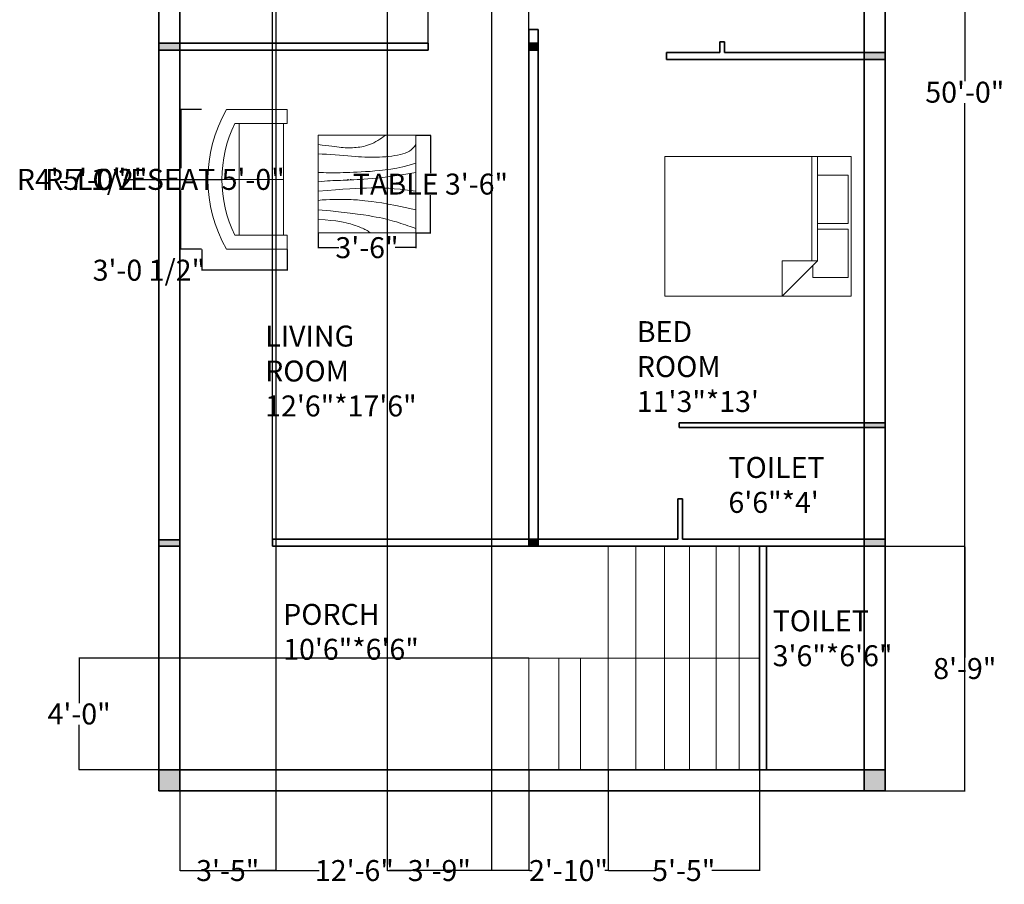
# Model space of a CAD drawing. Units: inches. Extents: x 23641 to 24129, y 27170 to 27889.
# Tile 1 of 2: x 23641 to 24064, y 27170 to 27541. Entities that reach past the tile are written whole.
import ezdxf

# ---------------------------------------------------------------- set-up
doc = ezdxf.new("R2010")
doc.units = ezdxf.units.IN
doc.header["$MEASUREMENT"] = 0
for name, color, linetype, lineweight in [('A-ANNO-DIMS', 2, 'Continuous', 18), ('A-AREA-IDEN', 7, 'Continuous', 25), ('A-FLOR-STRS', 7, 'Continuous', 18), ('A-FURN', 8, 'Continuous', 18), ('A-WALL', 7, 'Continuous', 35), ('A-WALL-PATT', 7, 'Continuous', 13)]:
    doc.layers.add(name, color=color, linetype=linetype, lineweight=lineweight)
doc.styles.get("Standard").update_dxf_attribs({"font": 'arial.ttf'})
doc.dimstyles.get("Standard").update_dxf_attribs({"dimtxt": 9, "dimasz": 0.18, "dimexe": 0.18, "dimexo": 0.0625, "dimgap": 0.09, "dimtad": 0, "dimtih": 1, "dimtoh": 1, "dimdec": 0, "dimzin": 0, "dimdsep": 46, "dimlunit": 3, "dimtxsty": 'Standard', "dimcen": 0.09, "dimadec": 0, "dimazin": 0, "dimtfac": 1, "dimtdec": 0, "dimtofl": 0, "dimtmove": 0, "dimatfit": 3, "dimfxl": 1, "dimtolj": 1, "dimtzin": 0, "dimarcsym": 0})

# ---------------------------------------------------------------- blocks, each defined once
blk = doc.blocks.new('Table - Square Woodgrain 42 x 42 in.')
blk.add_line((0, -42), (42, -42))
for points in [[(0, -4), (1.704, -4.2172), (3.2358, -4.4188), (4.615, -4.604), (5.8615, -4.7721), (6.9951, -4.9224), (8.0357, -5.0541), (9.0031, -5.1667), (9.9171, -5.2594), (10.7951, -5.3316), (11.6445, -5.3836), (12.4702, -5.4157), (13.277, -5.4283), (14.0698, -5.4217), (14.8535, -5.3964), (15.6331, -5.3526), (16.4133, -5.2908), (17.1986, -5.2103), (17.9913, -5.1062), (18.793, -4.9727), (19.6056, -4.8038), (20.4307, -4.5937), (21.2701, -4.3365), (22.1256, -4.0262), (22.9989, -3.6571), (23.888, -3.2272), (24.7756, -2.7516), (25.6408, -2.2491), (26.4624, -1.7387), (27.2195, -1.2395), (27.891, -0.7703), (28.456, -0.3501), (28.8934, 0.002)], [(0, -42), (0, 0), (42, 0), (42, -42)], [(0, -8), (1.8203, -8.1001), (3.6741, -8.2149), (5.5411, -8.3408), (7.4011, -8.4741), (9.2339, -8.6112), (11.0193, -8.7484), (12.7371, -8.8821), (14.3671, -9.0086), (15.8954, -9.1246), (17.3337, -9.2278), (18.6997, -9.3159), (20.0116, -9.387), (21.2871, -9.4389), (22.5442, -9.4696), (23.8008, -9.477), (25.0749, -9.459), (26.3791, -9.4137), (27.7049, -9.3403), (29.0383, -9.2382), (30.3655, -9.1068), (31.6728, -8.9455), (32.9461, -8.7535), (34.1717, -8.5304), (35.3358, -8.2756), (36.4268, -7.9863), (37.443, -7.6521), (38.3849, -7.2603), (39.253, -6.7986), (40.048, -6.2542), (40.7705, -5.6147), (41.421, -4.8674), (42, -4)], [(42, -12), (39.1784, -12.8621), (36.4519, -13.5654), (33.8246, -14.1294), (31.3004, -14.5731), (28.8832, -14.9161), (26.577, -15.1775), (24.3858, -15.3768), (22.3136, -15.5332), (20.3622, -15.6632), (18.5254, -15.7718), (16.7947, -15.8612), (15.1618, -15.9338), (13.6183, -15.9916), (12.1558, -16.0369), (10.7659, -16.0718), (9.4403, -16.0987), (8.1703, -16.1191), (6.9461, -16.1325), (5.7577, -16.1377), (4.595, -16.1335), (3.4479, -16.1188), (2.3064, -16.0924), (1.1604, -16.0532), (0, -16)], [(42, -16), (37.6529, -16.7365), (33.8802, -17.329), (30.6179, -17.7961), (27.8015, -18.1561), (25.3668, -18.4275), (23.2497, -18.6288), (21.3859, -18.7785), (19.7111, -18.8949), (18.1693, -18.9939), (16.7375, -19.0795), (15.401, -19.1534), (14.1449, -19.217), (12.9544, -19.2717), (11.8148, -19.3191), (10.7113, -19.3606), (9.6291, -19.3976), (8.5534, -19.4323), (7.47, -19.4689), (6.3643, -19.5122), (5.222, -19.5672), (4.0288, -19.6386), (2.7703, -19.7313), (1.4321, -19.8501), (0, -20)], [(0, -24), (3.9243, -23.6805), (7.4766, -23.4138), (10.6891, -23.1954), (13.5943, -23.0205), (16.2247, -22.8847), (18.6125, -22.7832), (20.7903, -22.7116), (22.7903, -22.6651), (24.6563, -22.642), (26.4764, -22.6507), (28.35, -22.7024), (30.3766, -22.8084), (32.6555, -22.98), (35.2861, -23.2283), (38.3678, -23.5645), (42, -24)], [(42, -32), (37.392, -31.017), (33.4585, -30.2231), (30.1291, -29.5949), (27.3334, -29.109), (25.0009, -28.742), (23.0612, -28.4707), (21.4439, -28.2716), (20.0786, -28.1215), (18.8998, -28.0002), (17.8609, -27.9014), (16.9206, -27.8219), (16.0371, -27.7588), (15.1691, -27.709), (14.2748, -27.6693), (13.3128, -27.6368), (12.2415, -27.6083), (11.0295, -27.5824), (9.6867, -27.5643), (8.233, -27.5608), (6.6884, -27.5787), (5.0728, -27.6248), (3.4062, -27.7058), (1.7086, -27.8286), (0, -28)], [(0, -32), (5.4026, -32.5358), (9.9494, -33.019), (13.7424, -33.4553), (16.8834, -33.8505), (19.4743, -34.2106), (21.6171, -34.5413), (23.4136, -34.8486), (24.9657, -35.1382), (26.3614, -35.4156), (27.6332, -35.6841), (28.7995, -35.9467), (29.8788, -36.2064), (30.8897, -36.4661), (31.8507, -36.7288), (32.7802, -36.9973), (33.6968, -37.2747), (34.6175, -37.5635), (35.5531, -37.8651), (36.5128, -38.1805), (37.506, -38.5108), (38.5421, -38.8568), (39.6302, -39.2197), (40.7797, -39.6004), (42, -40)], [(0, -36), (3.0098, -36.2857), (5.5354, -36.5643), (7.6368, -36.8359), (9.374, -37.1009), (10.807, -37.3597), (11.9957, -37.6126), (13.0002, -37.8599), (13.8804, -38.102), (14.6874, -38.3393), (15.4365, -38.5729), (16.1338, -38.8041), (16.7858, -39.0341), (17.3987, -39.264), (17.9787, -39.4952), (18.5322, -39.7288), (19.0655, -39.9662), (19.5832, -40.2081), (20.0842, -40.4544), (20.5657, -40.7046), (21.0249, -40.9581), (21.459, -41.2144), (21.8653, -41.4731), (22.2409, -41.7335), (22.5831, -41.9951)]]:
    blk.add_lwpolyline(points)
blk = doc.blocks.new('Sofa - Roundback Loveseat 5 ft.')
for p, q in [((0, -32.44198), (0, -5.99998)), ((-24, -33.99998), (-24, -11.46958)), ((24.00004, -33.99998), (24.00004, -11.46958)), ((-23.9998, -13.38178), (23.99986, -13.38178)), ((-24, -32.44198), (24.00004, -32.44198))]:
    blk.add_line(p, q)
for points in [[(-24, -33.99998), (-30, -33.99998), (-30, -7.99998)], [(30.00004, -7.99998), (30.00004, -33.99998), (24.00004, -33.99998)]]:
    blk.add_lwpolyline(points)
for centre, radius, start, end in [((0, -60.24998), 60.24998, 60.13715, 119.8628), ((0, -61.38438), 55.38444, 64.32083, 115.6792)]:
    blk.add_arc(centre, radius, start, end)
blk = doc.blocks.new('Bed - Queen')
for p, q in [((0, -80.00003), (0, 0)), ((0, 0), (59.99999, 0)), ((59.99999, 0), (59.99999, -80.00003)), ((7.99999, -1.2), (28.79998, -1.2)), ((7.99999, -14.4), (7.99999, -1.2)), ((28.79998, -1.2), (28.79998, -14.4)), ((31.19999, -1.2), (51.99999, -1.2)), ((31.19999, -14.4), (31.19999, -1.2)), ((51.99999, -1.2), (51.99999, -16.4)), ((0, -14.4), (44.8, -14.4)), ((44.8, -16.8), (0, -16.8)), ((59.99999, -29.6), (44.8, -14.4)), ((44.8, -14.4), (44.8, -29.6)), ((51.99999, -16.4), (46.79936, -16.4)), ((44.8, -29.6), (59.99999, -29.6)), ((59.99999, -80.00003), (0, -80.00003))]:
    blk.add_line(p, q)
blk = doc.blocks.new('*D17')
at = {"layer": 'A-ANNO-DIMS', "color": 0, "lineweight": -2, "transparency": 16777216}
for p, q in [((23811.46, 27491.81), (23817.87, 27491.81)), ((23817.69, 27491.63), (23817.69, 27475.5)), ((23817.69, 27449.99), (23817.69, 27466.12)), ((23811.46, 27449.81), (23817.87, 27449.81))]:
    blk.add_line(p, q, dxfattribs=at)
at = {"layer": 'A-ANNO-DIMS', "color": 0, "transparency": 16777216}
for points in [[(23817.66, 27491.63), (23817.72, 27491.63), (23817.69, 27491.81)], [(23817.66, 27449.99), (23817.72, 27449.99), (23817.69, 27449.81)]]:
    blk.add_solid(points, dxfattribs=at)
at = {"layer": 'Defpoints', "color": 0, "transparency": 16777216}
for p in [(23811.39, 27491.81), (23817.69, 27491.81), (23811.39, 27449.81)]:
    blk.add_point(p, dxfattribs=at)
at = {"layer": 'A-ANNO-DIMS', "color": 0, "transparency": 16777216, "insert": (23817.69, 27470.81), "char_height": 9, "attachment_point": 5}
blk.add_mtext('\\A1;TABLE 3\'-6"', dxfattribs=at)
blk = doc.blocks.new('*D18')
at = {"layer": 'A-ANNO-DIMS', "color": 0, "lineweight": -2, "transparency": 16777216}
for p, q in [((23769.39, 27449.74), (23769.39, 27443.33)), ((23811.39, 27449.74), (23811.39, 27443.33)), ((23769.57, 27443.51), (23778.34, 27443.51)), ((23811.21, 27443.51), (23802.44, 27443.51))]:
    blk.add_line(p, q, dxfattribs=at)
at = {"layer": 'A-ANNO-DIMS', "color": 0, "transparency": 16777216}
for points in [[(23769.57, 27443.54), (23769.57, 27443.48), (23769.39, 27443.51)], [(23811.21, 27443.54), (23811.21, 27443.48), (23811.39, 27443.51)]]:
    blk.add_solid(points, dxfattribs=at)
at = {"layer": 'Defpoints', "color": 0, "transparency": 16777216}
for p in [(23769.39, 27449.81), (23811.39, 27449.81), (23811.39, 27443.51)]:
    blk.add_point(p, dxfattribs=at)
at = {"layer": 'A-ANNO-DIMS', "color": 0, "transparency": 16777216, "insert": (23790.39, 27443.51), "char_height": 9, "attachment_point": 5}
blk.add_mtext('\\A1;3\'-6"', dxfattribs=at)
blk = doc.blocks.new('*D19')
at = {"layer": 'A-ANNO-DIMS', "color": 0, "lineweight": -2, "transparency": 16777216}
for p, q in [((23719.36, 27502.83), (23710.24, 27502.83)), ((23710.42, 27502.65), (23710.42, 27477.58)), ((23710.42, 27443.01), (23710.42, 27468.08)), ((23719.36, 27442.83), (23710.24, 27442.83))]:
    blk.add_line(p, q, dxfattribs=at)
at = {"layer": 'A-ANNO-DIMS', "color": 0, "transparency": 16777216}
for points in [[(23710.39, 27502.65), (23710.45, 27502.65), (23710.42, 27502.83)], [(23710.39, 27443.01), (23710.45, 27443.01), (23710.42, 27442.83)]]:
    blk.add_solid(points, dxfattribs=at)
at = {"layer": 'Defpoints', "color": 0, "transparency": 16777216}
for p in [(23710.42, 27502.83), (23719.42, 27502.83), (23719.42, 27442.83)]:
    blk.add_point(p, dxfattribs=at)
at = {"layer": 'A-ANNO-DIMS', "color": 0, "transparency": 16777216, "insert": (23710.42, 27472.83), "char_height": 9, "attachment_point": 5}
blk.add_mtext('\\A1;LOVESEAT 5\'-0"', dxfattribs=at)
blk = doc.blocks.new('*D20')
at = {"layer": 'A-ANNO-DIMS', "color": 0, "lineweight": -2, "transparency": 16777216}
for p, q in [((23719.42, 27442.77), (23719.42, 27433.65)), ((23756.08, 27442.77), (23756.08, 27433.65)), ((23719.42, 27433.83), (23719.24, 27433.83)), ((23755.9, 27433.83), (23719.6, 27433.83))]:
    blk.add_line(p, q, dxfattribs=at)
at = {"layer": 'A-ANNO-DIMS', "color": 0, "transparency": 16777216}
for points in [[(23719.6, 27433.86), (23719.6, 27433.8), (23719.42, 27433.83)], [(23755.9, 27433.86), (23755.9, 27433.8), (23756.08, 27433.83)]]:
    blk.add_solid(points, dxfattribs=at)
at = {"layer": 'Defpoints', "color": 0, "transparency": 16777216}
for p in [(23719.42, 27442.83), (23756.08, 27442.83), (23719.42, 27433.83)]:
    blk.add_point(p, dxfattribs=at)
at = {"layer": 'A-ANNO-DIMS', "color": 0, "transparency": 16777216, "insert": (23696.7, 27433.83), "char_height": 9, "attachment_point": 5}
blk.add_mtext('\\A1;3\'-0 1/2"', dxfattribs=at)
blk = doc.blocks.new('*D23')
at = {"layer": 'A-ANNO-DIMS', "color": 0, "lineweight": -2, "transparency": 16777216}
for p, q in [((24013.05, 27810.27), (24047.41, 27810.27)), ((24047.23, 27810.09), (24047.23, 27514.96)), ((24047.23, 27210.45), (24047.23, 27505.59)), ((24013.05, 27210.27), (24047.41, 27210.27))]:
    blk.add_line(p, q, dxfattribs=at)
at = {"layer": 'A-ANNO-DIMS', "color": 0, "transparency": 16777216}
for points in [[(24047.2, 27810.09), (24047.26, 27810.09), (24047.23, 27810.27)], [(24047.2, 27210.45), (24047.26, 27210.45), (24047.23, 27210.27)]]:
    blk.add_solid(points, dxfattribs=at)
at = {"layer": 'Defpoints', "color": 0, "transparency": 16777216}
for p in [(24012.98, 27810.27), (24047.23, 27810.27), (24012.98, 27210.27)]:
    blk.add_point(p, dxfattribs=at)
at = {"layer": 'A-ANNO-DIMS', "color": 0, "transparency": 16777216, "insert": (24047.23, 27510.27), "char_height": 9, "attachment_point": 5}
blk.add_mtext('\\A1;50\'-0"', dxfattribs=at)
blk = doc.blocks.new('*D25')
at = {"layer": 'A-ANNO-DIMS', "color": 0, "lineweight": -2, "transparency": 16777216}
for p, q in [((23709.98, 27315.33), (23709.98, 27844.7)), ((23710.16, 27844.52), (23717.83, 27844.52)), ((23749.6, 27844.52), (23741.93, 27844.52)), ((23749.78, 27315.33), (23749.78, 27844.7))]:
    blk.add_line(p, q, dxfattribs=at)
at = {"layer": 'A-ANNO-DIMS', "color": 0, "transparency": 16777216}
for points in [[(23710.16, 27844.55), (23710.16, 27844.49), (23709.98, 27844.52)], [(23749.6, 27844.55), (23749.6, 27844.49), (23749.78, 27844.52)]]:
    blk.add_solid(points, dxfattribs=at)
at = {"layer": 'Defpoints', "color": 0, "transparency": 16777216}
for p in [(23749.78, 27844.52), (23709.98, 27315.27), (23749.78, 27315.27)]:
    blk.add_point(p, dxfattribs=at)
at = {"layer": 'A-ANNO-DIMS', "color": 0, "transparency": 16777216, "insert": (23729.88, 27844.52), "char_height": 9, "attachment_point": 5}
blk.add_mtext('\\A1;3\'-4"', dxfattribs=at)
blk = doc.blocks.new('*D26')
at = {"layer": 'A-ANNO-DIMS', "color": 0, "lineweight": -2, "transparency": 16777216}
for p, q in [((24013.05, 27315.27), (24047.41, 27315.27)), ((24047.23, 27315.09), (24047.23, 27267.46)), ((24047.23, 27210.45), (24047.23, 27258.09)), ((24013.05, 27210.27), (24047.41, 27210.27))]:
    blk.add_line(p, q, dxfattribs=at)
at = {"layer": 'A-ANNO-DIMS', "color": 0, "transparency": 16777216}
for points in [[(24047.2, 27315.09), (24047.26, 27315.09), (24047.23, 27315.27)], [(24047.2, 27210.45), (24047.26, 27210.45), (24047.23, 27210.27)]]:
    blk.add_solid(points, dxfattribs=at)
at = {"layer": 'Defpoints', "color": 0, "transparency": 16777216}
for p in [(24012.98, 27315.27), (24047.23, 27315.27), (24012.98, 27210.27)]:
    blk.add_point(p, dxfattribs=at)
at = {"layer": 'A-ANNO-DIMS', "color": 0, "transparency": 16777216, "insert": (24047.23, 27262.77), "char_height": 9, "attachment_point": 5}
blk.add_mtext('\\A1;8\'-9"', dxfattribs=at)
blk = doc.blocks.new('*D27')
at = {"layer": 'A-ANNO-DIMS', "color": 0, "lineweight": -2, "transparency": 16777216}
for p, q in [((23893.98, 27219.21), (23893.98, 27175.84)), ((23958.98, 27219.21), (23958.98, 27175.84)), ((23894.16, 27176.02), (23914.43, 27176.02)), ((23958.8, 27176.02), (23938.54, 27176.02))]:
    blk.add_line(p, q, dxfattribs=at)
at = {"layer": 'A-ANNO-DIMS', "color": 0, "transparency": 16777216}
for points in [[(23894.16, 27176.05), (23894.16, 27175.99), (23893.98, 27176.02)], [(23958.8, 27176.05), (23958.8, 27175.99), (23958.98, 27176.02)]]:
    blk.add_solid(points, dxfattribs=at)
at = {"layer": 'Defpoints', "color": 0, "transparency": 16777216}
for p in [(23893.98, 27219.27), (23958.98, 27219.27), (23958.98, 27176.02)]:
    blk.add_point(p, dxfattribs=at)
at = {"layer": 'A-ANNO-DIMS', "color": 0, "transparency": 16777216, "insert": (23926.48, 27176.02), "char_height": 9, "attachment_point": 5}
blk.add_mtext('\\A1;5\'-5"', dxfattribs=at)
blk = doc.blocks.new('*D29')
at = {"layer": 'A-ANNO-DIMS', "color": 0, "lineweight": -2, "transparency": 16777216}
for p, q in [((23799.02, 27654.21), (23799.02, 27175.84)), ((23843.92, 27654.21), (23843.92, 27175.84)), ((23799.2, 27176.02), (23809.42, 27176.02)), ((23843.74, 27176.02), (23833.52, 27176.02))]:
    blk.add_line(p, q, dxfattribs=at)
at = {"layer": 'A-ANNO-DIMS', "color": 0, "transparency": 16777216}
for points in [[(23799.2, 27176.05), (23799.2, 27175.99), (23799.02, 27176.02)], [(23843.74, 27176.05), (23843.74, 27175.99), (23843.92, 27176.02)]]:
    blk.add_solid(points, dxfattribs=at)
at = {"layer": 'Defpoints', "color": 0, "transparency": 16777216}
for p in [(23799.02, 27654.27), (23843.92, 27654.27), (23843.92, 27176.02)]:
    blk.add_point(p, dxfattribs=at)
at = {"layer": 'A-ANNO-DIMS', "color": 0, "transparency": 16777216, "insert": (23821.47, 27176.02), "char_height": 9, "attachment_point": 5}
blk.add_mtext('\\A1;3\'-9"', dxfattribs=at)
blk = doc.blocks.new('*D30')
at = {"layer": 'A-ANNO-DIMS', "color": 0, "lineweight": -2, "transparency": 16777216}
for p, q in [((23709.98, 27657.21), (23709.98, 27175.84)), ((23751.17, 27657.21), (23751.17, 27175.84)), ((23710.16, 27176.02), (23718.53, 27176.02)), ((23750.99, 27176.02), (23742.63, 27176.02))]:
    blk.add_line(p, q, dxfattribs=at)
at = {"layer": 'A-ANNO-DIMS', "color": 0, "transparency": 16777216}
for points in [[(23710.16, 27176.05), (23710.16, 27175.99), (23709.98, 27176.02)], [(23750.99, 27176.05), (23750.99, 27175.99), (23751.17, 27176.02)]]:
    blk.add_solid(points, dxfattribs=at)
at = {"layer": 'Defpoints', "color": 0, "transparency": 16777216}
for p in [(23709.98, 27657.27), (23751.17, 27657.27), (23751.17, 27176.02)]:
    blk.add_point(p, dxfattribs=at)
at = {"layer": 'A-ANNO-DIMS', "color": 0, "transparency": 16777216, "insert": (23730.58, 27176.02), "char_height": 9, "attachment_point": 5}
blk.add_mtext('\\A1;3\'-5"', dxfattribs=at)
blk = doc.blocks.new('*D32')
at = {"layer": 'A-ANNO-DIMS', "color": 0, "lineweight": -2, "transparency": 16777216}
for p, q in [((23859.92, 27267.27), (23666.55, 27267.27)), ((23666.73, 27267.09), (23666.73, 27247.96)), ((23666.73, 27219.45), (23666.73, 27238.59)), ((23859.92, 27219.27), (23666.55, 27219.27))]:
    blk.add_line(p, q, dxfattribs=at)
at = {"layer": 'A-ANNO-DIMS', "color": 0, "transparency": 16777216}
for points in [[(23666.7, 27267.09), (23666.76, 27267.09), (23666.73, 27267.27)], [(23666.7, 27219.45), (23666.76, 27219.45), (23666.73, 27219.27)]]:
    blk.add_solid(points, dxfattribs=at)
at = {"layer": 'Defpoints', "color": 0, "transparency": 16777216}
for p in [(23666.73, 27267.27), (23859.98, 27267.27), (23859.98, 27219.27)]:
    blk.add_point(p, dxfattribs=at)
at = {"layer": 'A-ANNO-DIMS', "color": 0, "transparency": 16777216, "insert": (23666.73, 27243.27), "char_height": 9, "attachment_point": 5}
blk.add_mtext('\\A1;4\'-0"', dxfattribs=at)
blk = doc.blocks.new('*D33')
at = {"layer": 'A-ANNO-DIMS', "color": 0, "lineweight": -2, "transparency": 16777216}
for p, q in [((23859.98, 27219.21), (23859.98, 27175.84)), ((23893.98, 27219.21), (23893.98, 27175.84)), ((23860.16, 27176.02), (23861.36, 27176.02)), ((23893.8, 27176.02), (23892.61, 27176.02))]:
    blk.add_line(p, q, dxfattribs=at)
at = {"layer": 'A-ANNO-DIMS', "color": 0, "transparency": 16777216}
for points in [[(23860.16, 27176.05), (23860.16, 27175.99), (23859.98, 27176.02)], [(23893.8, 27176.05), (23893.8, 27175.99), (23893.98, 27176.02)]]:
    blk.add_solid(points, dxfattribs=at)
at = {"layer": 'Defpoints', "color": 0, "transparency": 16777216}
for p in [(23859.98, 27219.27), (23893.98, 27219.27), (23893.98, 27176.02)]:
    blk.add_point(p, dxfattribs=at)
at = {"layer": 'A-ANNO-DIMS', "color": 0, "transparency": 16777216, "insert": (23876.98, 27176.02), "char_height": 9, "attachment_point": 5}
blk.add_mtext('\\A1;2\'-10"', dxfattribs=at)
blk = doc.blocks.new('*D34')
at = {"layer": 'A-ANNO-DIMS', "color": 0, "lineweight": -2, "transparency": 16777216}
for p, q in [((23709.98, 27219.21), (23709.98, 27175.84)), ((23859.98, 27219.21), (23859.98, 27175.84)), ((23710.16, 27176.02), (23769.86, 27176.02)), ((23859.8, 27176.02), (23800.11, 27176.02))]:
    blk.add_line(p, q, dxfattribs=at)
at = {"layer": 'A-ANNO-DIMS', "color": 0, "transparency": 16777216}
for points in [[(23710.16, 27176.05), (23710.16, 27175.99), (23709.98, 27176.02)], [(23859.8, 27176.05), (23859.8, 27175.99), (23859.98, 27176.02)]]:
    blk.add_solid(points, dxfattribs=at)
at = {"layer": 'Defpoints', "color": 0, "transparency": 16777216}
for p in [(23709.98, 27219.27), (23859.98, 27219.27), (23859.98, 27176.02)]:
    blk.add_point(p, dxfattribs=at)
at = {"layer": 'A-ANNO-DIMS', "color": 0, "transparency": 16777216, "insert": (23784.98, 27176.02), "char_height": 9, "attachment_point": 5}
blk.add_mtext('\\A1;12\'-6"', dxfattribs=at)
blk = doc.blocks.new('*D35')
at = {"layer": 'A-ANNO-DIMS', "color": 0, "lineweight": -2, "transparency": 16777216}
for p, q in [((23816.62, 27531.33), (23816.62, 27844.7)), ((23816.8, 27844.52), (23859.8, 27844.52)), ((23859.98, 27531.33), (23859.98, 27844.7)), ((23859.98, 27844.52), (23860.16, 27844.52))]:
    blk.add_line(p, q, dxfattribs=at)
at = {"layer": 'A-ANNO-DIMS', "color": 0, "transparency": 16777216}
for points in [[(23816.8, 27844.55), (23816.8, 27844.49), (23816.62, 27844.52)], [(23859.8, 27844.55), (23859.8, 27844.49), (23859.98, 27844.52)]]:
    blk.add_solid(points, dxfattribs=at)
at = {"layer": 'Defpoints', "color": 0, "transparency": 16777216}
for p in [(23859.98, 27844.52), (23816.62, 27531.27), (23859.98, 27531.27)]:
    blk.add_point(p, dxfattribs=at)
at = {"layer": 'A-ANNO-DIMS', "color": 0, "transparency": 16777216, "insert": (23882.7, 27844.52), "char_height": 9, "attachment_point": 5}
blk.add_mtext('\\A1;3\'-7 1/2"', dxfattribs=at)
blk = doc.blocks.new('*D36')
at = {"layer": 'A-ANNO-DIMS', "color": 0, "lineweight": -2, "transparency": 16777216}
for p, q in [((23685.94, 27472.83), (23721.91, 27472.83)), ((23782.24, 27472.83), (23782.42, 27472.83)), ((23782.33, 27472.74), (23782.33, 27472.92))]:
    blk.add_line(p, q, dxfattribs=at)
at = {"layer": 'A-ANNO-DIMS', "color": 0, "transparency": 16777216}
blk.add_solid([(23721.91, 27472.86), (23721.91, 27472.8), (23722.09, 27472.83)], dxfattribs=at)
at = {"layer": 'Defpoints', "color": 0, "transparency": 16777216}
for p in [(23722.09, 27472.83), (23782.33, 27472.83)]:
    blk.add_point(p, dxfattribs=at)
at = {"layer": 'A-ANNO-DIMS', "color": 0, "transparency": 16777216, "insert": (23669.58, 27472.83), "char_height": 9, "attachment_point": 5}
blk.add_mtext('\\A1;R5\'-0"', dxfattribs=at)
blk = doc.blocks.new('*D37')
at = {"layer": 'A-ANNO-DIMS', "color": 0, "lineweight": -2, "transparency": 16777216}
for p, q in [((23694.85, 27472.83), (23727.9, 27472.83)), ((23783.38, 27472.83), (23783.56, 27472.83)), ((23783.47, 27472.74), (23783.47, 27472.92))]:
    blk.add_line(p, q, dxfattribs=at)
at = {"layer": 'A-ANNO-DIMS', "color": 0, "transparency": 16777216}
blk.add_solid([(23727.9, 27472.86), (23727.9, 27472.8), (23728.08, 27472.83)], dxfattribs=at)
at = {"layer": 'Defpoints', "color": 0, "transparency": 16777216}
for p in [(23728.08, 27472.83), (23783.47, 27472.83)]:
    blk.add_point(p, dxfattribs=at)
at = {"layer": 'A-ANNO-DIMS', "color": 0, "transparency": 16777216, "insert": (23668.01, 27472.83), "char_height": 9, "attachment_point": 5}
blk.add_mtext('\\A1;R4\'-7 1/2"', dxfattribs=at)

msp = doc.modelspace()

# ---------------------------------------------------------------- hatches: boundary and pattern name
at = {"layer": 'A-WALL-PATT'}
h = msp.add_hatch(color=256, dxfattribs=at)
h.dxf.hatch_style = 1
h.paths.add_polyline_path([(23709.98, 27531.27), (23700.98, 27531.27), (23700.98, 27528.27), (23709.98, 27528.27)])
h = msp.add_hatch(color=256, dxfattribs=at)
h.dxf.hatch_style = 1
h.paths.add_polyline_path([(23863.98, 27531.27), (23859.98, 27531.27), (23859.98, 27528.27), (23863.98, 27528.27)])
h = msp.add_hatch(color=256, dxfattribs=at)
h.dxf.hatch_style = 1
h.paths.add_polyline_path([(24012.98, 27527.27), (24003.98, 27527.27), (24003.98, 27524.27), (24012.98, 27524.27)])
h = msp.add_hatch(color=256, dxfattribs=at)
h.dxf.hatch_style = 1
h.paths.add_polyline_path([(24012.98, 27368.27), (24003.98, 27368.27), (24003.98, 27366.27), (24012.98, 27366.27)])
h = msp.add_hatch(color=256, dxfattribs=at)
h.dxf.hatch_style = 1
h.paths.add_polyline_path([(23709.98, 27318.04), (23700.98, 27318.04), (23700.98, 27315.27), (23709.98, 27315.27)])
h = msp.add_hatch(color=256, dxfattribs=at)
h.dxf.hatch_style = 1
h.paths.add_polyline_path([(23863.98, 27318.27), (23859.98, 27318.27), (23859.98, 27315.27), (23863.98, 27315.27)])
h = msp.add_hatch(color=256, dxfattribs=at)
h.dxf.hatch_style = 1
h.paths.add_polyline_path([(24012.98, 27318.27), (24003.98, 27318.27), (24003.98, 27315.27), (24012.98, 27315.27)])
h = msp.add_hatch(color=256, dxfattribs=at)
h.dxf.hatch_style = 1
h.paths.add_polyline_path([(23709.98, 27219.27), (23700.98, 27219.27), (23700.98, 27210.27), (23709.98, 27210.27)])
h = msp.add_hatch(color=256, dxfattribs=at)
h.dxf.hatch_style = 1
h.paths.add_polyline_path([(24012.98, 27219.27), (24003.98, 27219.27), (24003.98, 27210.27), (24012.98, 27210.27)])

# ---------------------------------------------------------------- linework, layer by layer
at = {"layer": 'A-FLOR-STRS'}
for p, q in [((23893.98, 27315.27), (23893.98, 27219.27)), ((23905.85, 27315.27), (23905.85, 27219.27)), ((23918.2, 27315.27), (23918.2, 27219.27)), ((23928.97, 27315.27), (23928.97, 27219.27)), ((23940.42, 27315.27), (23940.42, 27219.27)), ((23950.3, 27315.27), (23950.3, 27219.27)), ((23859.98, 27267.27), (23859.98, 27219.27)), ((23859.98, 27267.27), (23958.98, 27267.27)), ((23872.76, 27267.27), (23872.76, 27219.27)), ((23882.16, 27267.27), (23882.16, 27219.27))]:
    msp.add_line(p, q, dxfattribs=at)
at = {"layer": 'A-WALL'}
for p, q in [((23709.98, 27531.27), (23709.98, 27654.27)), ((24003.98, 27602.27), (24003.98, 27527.27)), ((23859.98, 27528.27), (23859.98, 27537.13)), ((23859.98, 27537.13), (23863.98, 27537.13)), ((23863.98, 27537.13), (23863.98, 27531.27)), ((23709.98, 27531.27), (23700.98, 27531.27)), ((23709.98, 27531.27), (23816.62, 27531.27)), ((23709.98, 27531.27), (23709.98, 27528.27)), ((23816.62, 27531.27), (23816.62, 27528.27)), ((23859.98, 27531.27), (23863.98, 27531.27)), ((23863.98, 27531.27), (23863.98, 27528.27)), ((23941.98, 27531.97), (23943.98, 27531.97)), ((23941.98, 27531.97), (23941.98, 27527.27)), ((23943.98, 27531.97), (23943.98, 27527.27)), ((23709.98, 27528.27), (23700.98, 27528.27)), ((23709.98, 27528.27), (23816.62, 27528.27)), ((23709.98, 27219.27), (23709.98, 27528.27)), ((23859.98, 27528.27), (23859.98, 27315.27)), ((23859.98, 27528.27), (23863.98, 27528.27)), ((23863.98, 27528.27), (23863.98, 27315.27)), ((23919.11, 27527.27), (23919.11, 27524.27)), ((23919.11, 27527.27), (23941.98, 27527.27)), ((23943.98, 27527.27), (24003.98, 27527.27)), ((24003.98, 27527.27), (24012.98, 27527.27)), ((24003.98, 27524.27), (24003.98, 27527.27)), ((23919.11, 27524.27), (24003.98, 27524.27)), ((24003.98, 27524.27), (24003.98, 27368.27)), ((24003.98, 27524.27), (24012.98, 27524.27)), ((23924.47, 27368.27), (23924.47, 27366.27)), ((23924.47, 27368.27), (24003.98, 27368.27)), ((23924.47, 27366.27), (24003.98, 27366.27)), ((24003.98, 27366.27), (24003.98, 27368.27)), ((24003.98, 27368.27), (24012.98, 27368.27)), ((24003.98, 27366.27), (24003.98, 27318.27)), ((24003.98, 27366.27), (24012.98, 27366.27)), ((23923.98, 27335.63), (23923.98, 27318.27)), ((23923.98, 27335.63), (23925.98, 27335.63)), ((23925.98, 27335.63), (23925.98, 27318.27)), ((23709.98, 27318.04), (23700.98, 27318.04)), ((23749.78, 27318.27), (23863.98, 27318.27)), ((23749.78, 27318.27), (23749.78, 27315.27)), ((23863.98, 27318.27), (23923.98, 27318.27)), ((23925.98, 27318.27), (24003.98, 27318.27)), ((24003.98, 27318.27), (24012.98, 27318.27)), ((24003.98, 27315.27), (24003.98, 27318.27)), ((23700.98, 27315.27), (23709.98, 27315.27)), ((23709.98, 27219.27), (23709.98, 27315.27)), ((23749.78, 27315.27), (23863.98, 27315.27)), ((23863.98, 27315.27), (24003.98, 27315.27)), ((23958.98, 27315.27), (23958.98, 27219.27)), ((23961.98, 27315.27), (23961.98, 27219.27)), ((24003.98, 27315.27), (24003.98, 27219.27)), ((24003.98, 27315.27), (24012.98, 27315.27)), ((23709.98, 27219.27), (23700.98, 27219.27)), ((24003.98, 27219.27), (23709.98, 27219.27)), ((23709.98, 27219.27), (23709.98, 27210.27)), ((24003.98, 27219.27), (24012.98, 27219.27)), ((24003.98, 27219.27), (24003.98, 27210.27))]:
    msp.add_line(p, q, dxfattribs=at)
msp.add_lwpolyline([(23859.98, 27810.27), (24012.98, 27810.27), (24012.98, 27210.27), (23700.98, 27210.27), (23700.98, 27810.27), (23806.55, 27810.27)], dxfattribs=at)

# ---------------------------------------------------------------- block references
at = {"layer": 'A-FURN'}
for name, p, rotation in [('Sofa - Roundback Loveseat 5 ft.', (23722.09, 27472.83), 90), ('Bed - Queen', (23998.35, 27482.7), 270)]:
    msp.add_blockref(name, p, dxfattribs=dict(at, rotation=rotation))
msp.add_blockref('Table - Square Woodgrain 42 x 42 in.', (23769.39, 27491.81), dxfattribs=at)

# ---------------------------------------------------------------- texts
at = {"layer": 'A-AREA-IDEN', "char_height": 9, "attachment_point": 1}
for s, insert in [('BED ROOM\\P11\'3"*13\'', (23906.32, 27411.95)), ('LIVING ROOM\\P12\'6"*17\'6"', (23746.65, 27410.04)), ('TOILET\\P6\'6"*4\'', (23945.68, 27353.63)), ('PORCH\\P10\'6"*6\'6"', (23754.39, 27290.53)), ('TOILET\\P3\'6"*6\'6"', (23964.69, 27287.77))]:
    msp.add_mtext_dynamic_manual_height_columns(s, width=25.8959, gutter_width=1, heights=[0], dxfattribs=dict(at, insert=insert))

# ---------------------------------------------------------------- dimensions: what is measured, and where the dimension line sits
at = {"layer": 'A-ANNO-DIMS'}
for base, p1, p2, picture, middle in [((23859.98, 27844.52), (23816.62, 27531.27), (23859.98, 27531.27), '*D35', (23882.7, 27844.52)), ((23749.78, 27844.52), (23709.98, 27315.27), (23749.78, 27315.27), '*D25', (23729.88, 27844.52)), ((23751.17, 27176.02), (23709.98, 27657.27), (23751.17, 27657.27), '*D30', (23730.58, 27176.02)), ((23843.92, 27176.02), (23799.02, 27654.27), (23843.92, 27654.27), '*D29', (23821.47, 27176.02)), ((23811.39, 27443.51), (23769.39, 27449.81), (23811.39, 27449.81), '*D18', (23790.39, 27443.51)), ((23859.98, 27176.02), (23709.98, 27219.27), (23859.98, 27219.27), '*D34', (23784.98, 27176.02)), ((23893.98, 27176.02), (23859.98, 27219.27), (23893.98, 27219.27), '*D33', (23876.98, 27176.02)), ((23958.98, 27176.02), (23893.98, 27219.27), (23958.98, 27219.27), '*D27', (23926.48, 27176.02))]:
    dim = msp.add_linear_dim(base=base, p1=p1, p2=p2, dimstyle='Standard', override={"dimdec": 1, "dimlfac": 1, "dimrnd": 0, "dimzin": 1, "dimdsep": 46, "dimlunit": 4, "dimfrac": 2}, dxfattribs=at)
    dim.commit()
    dim.dimension.update_dxf_attribs({"geometry": picture, "text_midpoint": middle})
for base, p1, p2, angle, picture, middle in [((24047.23, 27810.27), (24012.98, 27210.27), (24012.98, 27810.27), 90, '*D23', (24047.23, 27510.27)), ((23719.42, 27433.83), (23756.08, 27442.83), (23719.42, 27442.83), 180, '*D20', (23696.7, 27433.83)), ((24047.23, 27315.27), (24012.98, 27210.27), (24012.98, 27315.27), 90, '*D26', (24047.23, 27262.77)), ((23666.73, 27267.27), (23859.98, 27219.27), (23859.98, 27267.27), 90, '*D32', (23666.73, 27243.27))]:
    dim = msp.add_linear_dim(base=base, p1=p1, p2=p2, angle=angle, dimstyle='Standard', override={"dimdec": 1, "dimlfac": 1, "dimrnd": 0, "dimzin": 1, "dimdsep": 46, "dimlunit": 4, "dimfrac": 2}, dxfattribs=at)
    dim.commit()
    dim.dimension.update_dxf_attribs({"geometry": picture, "text_midpoint": middle})
for base, p1, p2, text, picture, middle in [((23710.42, 27502.83), (23719.42, 27442.83), (23719.42, 27502.83), 'LOVESEAT <>', '*D19', (23710.42, 27472.83)), ((23817.69, 27491.81), (23811.39, 27449.81), (23811.39, 27491.81), 'TABLE <>', '*D17', (23817.69, 27470.81))]:
    dim = msp.add_linear_dim(base=base, p1=p1, p2=p2, angle=90, text=text, dimstyle='Standard', override={"dimdec": 1, "dimlfac": 1, "dimrnd": 0, "dimzin": 1, "dimdsep": 46, "dimlunit": 4, "dimfrac": 2}, dxfattribs=at)
    dim.commit()
    dim.dimension.update_dxf_attribs({"geometry": picture, "text_midpoint": middle})
for center, mpoint, picture, middle in [((23783.47, 27472.83), (23728.08, 27472.83), '*D37', (23694.85, 27472.83)), ((23782.33, 27472.83), (23722.09, 27472.83), '*D36', (23685.94, 27472.83))]:
    dim = msp.add_radius_dim(center=center, mpoint=mpoint, dimstyle='Standard', override={"dimdec": 1, "dimlfac": 1, "dimrnd": 0, "dimzin": 1, "dimdsep": 46, "dimlunit": 4, "dimfrac": 2}, dxfattribs=at)
    dim.commit()
    dim.dimension.update_dxf_attribs({"geometry": picture, "text_midpoint": middle, "dimtype": 164})

doc.saveas('drawing.dxf')
